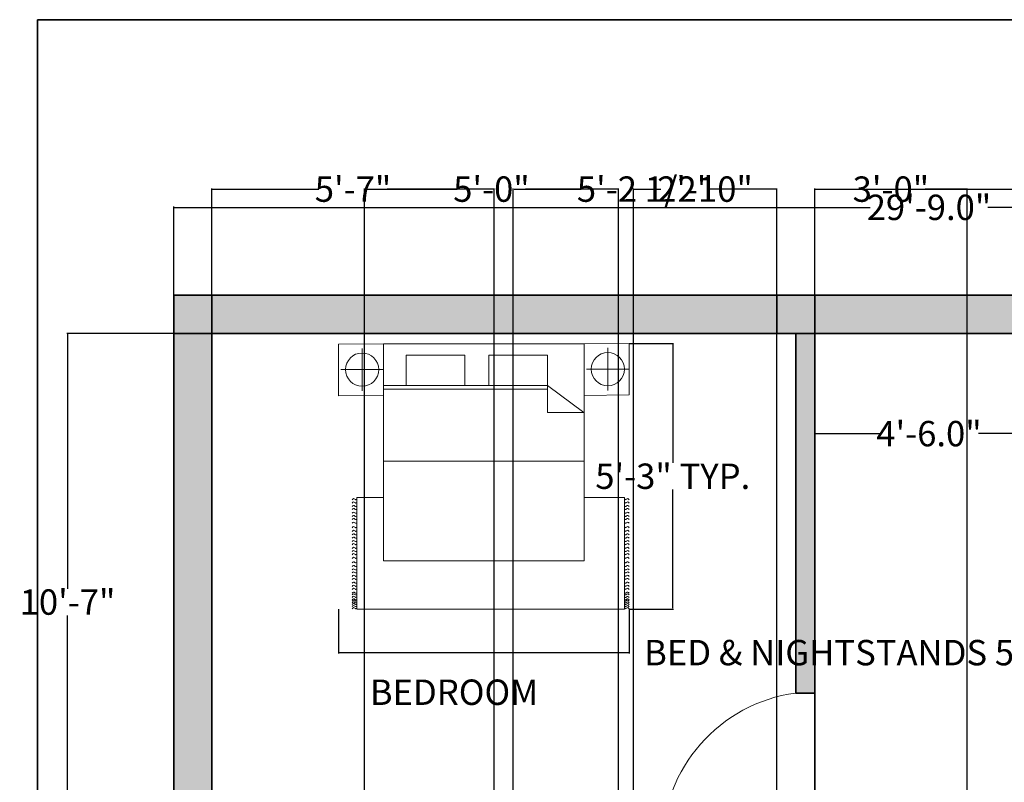
# Model space of a CAD drawing. Units: inches. Extents: x 74 to 548, y 68 to 649.
# Tile 5 of 6: x 79 to 311, y 469 to 649. Entities that reach past the tile are written whole.
import ezdxf

# ---------------------------------------------------------------- set-up
doc = ezdxf.new("R2010")
doc.units = ezdxf.units.IN
doc.header["$MEASUREMENT"] = 0
for name, color, linetype, lineweight in [('A-ANNO-DIMS', 2, 'Continuous', 18), ('A-ANNO-TTLB', 7, 'Continuous', 35), ('A-AREA-IDEN', 7, 'Continuous', 25), ('A-COLS', 7, 'Continuous', 35), ('A-DOOR', 3, 'Continuous', 18), ('A-FURN', 8, 'Continuous', 18), ('A-WALL', 7, 'Continuous', 35)]:
    doc.layers.add(name, color=color, linetype=linetype, lineweight=lineweight)
doc.layers.add('A-COLS-PATT', color=11, linetype='Continuous', lineweight=13, true_color=0xf27172)
doc.layers.add('A-WALL-PATT', color=7, linetype='Continuous', lineweight=13, true_color=0xffffff)
doc.styles.get("Standard").update_dxf_attribs({"font": 'arial.ttf'})
doc.dimstyles.get("Standard").update_dxf_attribs({"dimtxt": 6, "dimasz": 0.18, "dimexe": 0.18, "dimexo": 0.0625, "dimgap": 0.09, "dimtad": 0, "dimtih": 1, "dimtoh": 1, "dimdec": 1, "dimzin": 0, "dimdsep": 46, "dimlunit": 3, "dimtxsty": 'Standard', "dimcen": 0.09, "dimadec": 0, "dimazin": 0, "dimtfac": 1, "dimtdec": 1, "dimtofl": 0, "dimtmove": 0, "dimatfit": 3, "dimfxl": 1, "dimtolj": 1, "dimtzin": 0, "dimarcsym": 0})

# ---------------------------------------------------------------- blocks, each defined once
blk = doc.blocks.new('*D3')
at = {"layer": 'A-ANNO-DIMS', "color": 0, "lineweight": -2, "transparency": 16777216}
for p, q in [((114.96, 584.31), (114.96, 605.21)), ((471.96, 584.31), (471.96, 605.21)), ((115.14, 605.03), (279.52, 605.03)), ((471.78, 605.03), (307.4, 605.03))]:
    blk.add_line(p, q, dxfattribs=at)
at = {"layer": 'A-ANNO-DIMS', "color": 0, "transparency": 16777216}
for points in [[(115.14, 605.06), (115.14, 605), (114.96, 605.03)], [(471.78, 605.06), (471.78, 605), (471.96, 605.03)]]:
    blk.add_solid(points, dxfattribs=at)
at = {"layer": 'Defpoints', "color": 0, "transparency": 16777216}
for p in [(471.96, 605.03), (114.96, 584.24), (471.96, 584.24)]:
    blk.add_point(p, dxfattribs=at)
at = {"layer": 'A-ANNO-DIMS', "color": 0, "transparency": 16777216, "insert": (293.46, 605.03), "char_height": 6, "attachment_point": 5}
blk.add_mtext('\\A1;29\'-9.0"', dxfattribs=at)
blk = doc.blocks.new('*D5')
at = {"layer": 'A-ANNO-DIMS', "color": 0, "lineweight": -2, "transparency": 16777216}
for p, q in [((266.46, 561.7), (266.46, 551.37)), ((320.46, 559.19), (320.46, 551.37)), ((266.64, 551.55), (281.78, 551.55)), ((320.28, 551.55), (305.14, 551.55))]:
    blk.add_line(p, q, dxfattribs=at)
at = {"layer": 'A-ANNO-DIMS', "color": 0, "transparency": 16777216}
for points in [[(266.64, 551.58), (266.64, 551.52), (266.46, 551.55)], [(320.28, 551.58), (320.28, 551.52), (320.46, 551.55)]]:
    blk.add_solid(points, dxfattribs=at)
at = {"layer": 'Defpoints', "color": 0, "transparency": 16777216}
for p in [(266.46, 561.76), (320.46, 559.25), (320.46, 551.55)]:
    blk.add_point(p, dxfattribs=at)
at = {"layer": 'A-ANNO-DIMS', "color": 0, "transparency": 16777216, "insert": (293.46, 551.55), "char_height": 6, "attachment_point": 5}
blk.add_mtext('\\A1;4\'-6.0"', dxfattribs=at)
blk = doc.blocks.new('BED-DOUBLE-NIGHTSTANDS')
for p, q in [((-5.03, -1.07), (-5.03, -11.12)), ((53.03, -0.96), (53.03, -11.02)), ((0, -6.09), (-10.05, -6.09)), ((58.05, -5.99), (48, -5.99)), ((38.76, -9.86), (0, -9.86)), ((38.82, -10.68), (0, -10.68)), ((38.76, -9.86), (47.38, -16.22)), ((38.82, -9.86), (38.82, -16.22)), ((38.82, -16.22), (47.38, -16.22)), ((47.43, -27.72), (0, -27.72)), ((-6.27, -62.68), (-6.27, -36.31)), ((-6.27, -36.31), (0.03, -36.31)), ((47.43, -36.31), (56.97, -36.31)), ((56.97, -36.31), (56.97, -62.68)), ((56.97, -62.68), (-6.27, -62.68))]:
    blk.add_line(p, q)
for points in [[(-10.63, -12.29), (0, -12.19), (0, 0), (-10.63, -0.1)], [(47.43, 0), (47.43, -51.32), (0, -51.32), (0, 0)], [(47.43, -12.19), (58.05, -12.08), (58.05, 0.1), (47.43, 0)], [(19.25, -2.7), (19.25, -9.86), (5.36, -9.86), (5.36, -2.7)], [(38.82, -2.7), (38.82, -9.86), (24.92, -9.86), (24.92, -2.7)]]:
    blk.add_lwpolyline(points, close=True)
for centre in [(-5.03, -6.09), (53.03, -5.99)]:
    blk.add_circle(centre, 3.92)
for points, knots in [([(-7.4, -36.85), (-7.3, -36.72), (-7.11, -36.49), (-6.77, -36.72), (-6.49, -36.9), (-6.34, -36.79), (-6.27, -36.74)], [0, 0, 0, 0, 0.400747, 0.791423, 1.067667, 1.29709, 1.29709, 1.29709, 1.29709]), ([(58.08, -36.85), (57.99, -36.72), (57.8, -36.49), (57.45, -36.72), (57.17, -36.9), (57.02, -36.79), (56.96, -36.74)], [0, 0, 0, 0, 0.400747, 0.791423, 1.067667, 1.29709, 1.29709, 1.29709, 1.29709]), ([(-7.4, -37.62), (-7.3, -37.5), (-7.11, -37.26), (-6.77, -37.5), (-6.49, -37.68), (-6.34, -37.57), (-6.27, -37.52)], [0, 0, 0, 0, 0.400747, 0.791423, 1.067667, 1.29709, 1.29709, 1.29709, 1.29709]), ([(-7.4, -38.44), (-7.3, -38.32), (-7.11, -38.08), (-6.77, -38.32), (-6.49, -38.49), (-6.34, -38.39), (-6.27, -38.34)], [0, 0, 0, 0, 0.400747, 0.791423, 1.067667, 1.29709, 1.29709, 1.29709, 1.29709]), ([(-7.4, -39.17), (-7.3, -39.05), (-7.11, -38.81), (-6.77, -39.05), (-6.49, -39.22), (-6.34, -39.11), (-6.27, -39.07)], [0, 0, 0, 0, 0.400747, 0.791423, 1.067667, 1.29709, 1.29709, 1.29709, 1.29709]), ([(58.08, -37.62), (57.99, -37.5), (57.8, -37.26), (57.45, -37.5), (57.17, -37.68), (57.02, -37.57), (56.96, -37.52)], [0, 0, 0, 0, 0.400747, 0.791423, 1.067667, 1.29709, 1.29709, 1.29709, 1.29709]), ([(58.08, -38.44), (57.99, -38.32), (57.8, -38.08), (57.45, -38.32), (57.17, -38.49), (57.02, -38.39), (56.96, -38.34)], [0, 0, 0, 0, 0.400747, 0.791423, 1.067667, 1.29709, 1.29709, 1.29709, 1.29709]), ([(58.08, -39.17), (57.99, -39.05), (57.8, -38.81), (57.45, -39.05), (57.17, -39.22), (57.02, -39.11), (56.96, -39.07)], [0, 0, 0, 0, 0.400747, 0.791423, 1.067667, 1.29709, 1.29709, 1.29709, 1.29709]), ([(-7.4, -40.05), (-7.3, -39.93), (-7.11, -39.69), (-6.77, -39.93), (-6.49, -40.1), (-6.34, -40), (-6.27, -39.95)], [0, 0, 0, 0, 0.400747, 0.791423, 1.067667, 1.29709, 1.29709, 1.29709, 1.29709]), ([(-7.4, -40.8), (-7.3, -40.68), (-7.11, -40.44), (-6.77, -40.68), (-6.49, -40.85), (-6.34, -40.75), (-6.27, -40.7)], [0, 0, 0, 0, 0.400747, 0.791423, 1.067667, 1.29709, 1.29709, 1.29709, 1.29709]), ([(-7.4, -41.53), (-7.3, -41.41), (-7.11, -41.17), (-6.77, -41.41), (-6.49, -41.58), (-6.34, -41.48), (-6.27, -41.43)], [0, 0, 0, 0, 0.400747, 0.791423, 1.067667, 1.29709, 1.29709, 1.29709, 1.29709]), ([(58.08, -40.05), (57.99, -39.93), (57.8, -39.69), (57.45, -39.93), (57.17, -40.1), (57.02, -40), (56.96, -39.95)], [0, 0, 0, 0, 0.400747, 0.791423, 1.067667, 1.29709, 1.29709, 1.29709, 1.29709]), ([(58.08, -40.8), (57.99, -40.68), (57.8, -40.44), (57.45, -40.68), (57.17, -40.85), (57.02, -40.75), (56.96, -40.7)], [0, 0, 0, 0, 0.400747, 0.791423, 1.067667, 1.29709, 1.29709, 1.29709, 1.29709]), ([(58.08, -41.53), (57.99, -41.41), (57.8, -41.17), (57.45, -41.41), (57.17, -41.58), (57.02, -41.48), (56.96, -41.43)], [0, 0, 0, 0, 0.400747, 0.791423, 1.067667, 1.29709, 1.29709, 1.29709, 1.29709]), ([(-7.4, -42.41), (-7.3, -42.29), (-7.11, -42.05), (-6.77, -42.29), (-6.49, -42.46), (-6.34, -42.36), (-6.27, -42.31)], [0, 0, 0, 0, 0.400747, 0.791423, 1.067667, 1.29709, 1.29709, 1.29709, 1.29709]), ([(-7.4, -43.45), (-7.3, -43.33), (-7.11, -43.09), (-6.77, -43.33), (-6.49, -43.5), (-6.34, -43.39), (-6.27, -43.35)], [0, 0, 0, 0, 0.400747, 0.791423, 1.067667, 1.29709, 1.29709, 1.29709, 1.29709]), ([(-7.4, -44.33), (-7.3, -44.21), (-7.11, -43.97), (-6.77, -44.21), (-6.49, -44.38), (-6.34, -44.28), (-6.27, -44.23)], [0, 0, 0, 0, 0.400747, 0.791423, 1.067667, 1.29709, 1.29709, 1.29709, 1.29709]), ([(58.08, -42.41), (57.99, -42.29), (57.8, -42.05), (57.45, -42.29), (57.17, -42.46), (57.02, -42.36), (56.96, -42.31)], [0, 0, 0, 0, 0.400747, 0.791423, 1.067667, 1.29709, 1.29709, 1.29709, 1.29709]), ([(58.08, -43.45), (57.99, -43.33), (57.8, -43.09), (57.45, -43.33), (57.17, -43.5), (57.02, -43.39), (56.96, -43.35)], [0, 0, 0, 0, 0.400747, 0.791423, 1.067667, 1.29709, 1.29709, 1.29709, 1.29709]), ([(58.08, -44.33), (57.99, -44.21), (57.8, -43.97), (57.45, -44.21), (57.17, -44.38), (57.02, -44.28), (56.96, -44.23)], [0, 0, 0, 0, 0.400747, 0.791423, 1.067667, 1.29709, 1.29709, 1.29709, 1.29709]), ([(-7.4, -45.15), (-7.3, -45.03), (-7.11, -44.79), (-6.77, -45.03), (-6.49, -45.2), (-6.34, -45.09), (-6.27, -45.05)], [0, 0, 0, 0, 0.400747, 0.791423, 1.067667, 1.29709, 1.29709, 1.29709, 1.29709]), ([(-7.4, -45.92), (-7.3, -45.8), (-7.11, -45.56), (-6.77, -45.8), (-6.49, -45.98), (-6.34, -45.87), (-6.27, -45.82)], [0, 0, 0, 0, 0.400747, 0.791423, 1.067667, 1.29709, 1.29709, 1.29709, 1.29709]), ([(-7.4, -46.74), (-7.3, -46.62), (-7.11, -46.38), (-6.77, -46.62), (-6.49, -46.79), (-6.34, -46.69), (-6.27, -46.64)], [0, 0, 0, 0, 0.400747, 0.791423, 1.067667, 1.29709, 1.29709, 1.29709, 1.29709]), ([(58.08, -45.15), (57.99, -45.03), (57.8, -44.79), (57.45, -45.03), (57.17, -45.2), (57.02, -45.09), (56.96, -45.05)], [0, 0, 0, 0, 0.400747, 0.791423, 1.067667, 1.29709, 1.29709, 1.29709, 1.29709]), ([(58.08, -45.92), (57.99, -45.8), (57.8, -45.56), (57.45, -45.8), (57.17, -45.98), (57.02, -45.87), (56.96, -45.82)], [0, 0, 0, 0, 0.400747, 0.791423, 1.067667, 1.29709, 1.29709, 1.29709, 1.29709]), ([(58.08, -46.74), (57.99, -46.62), (57.8, -46.38), (57.45, -46.62), (57.17, -46.79), (57.02, -46.69), (56.96, -46.64)], [0, 0, 0, 0, 0.400747, 0.791423, 1.067667, 1.29709, 1.29709, 1.29709, 1.29709]), ([(-7.4, -47.47), (-7.3, -47.35), (-7.11, -47.11), (-6.77, -47.35), (-6.49, -47.52), (-6.34, -47.41), (-6.27, -47.37)], [0, 0, 0, 0, 0.400747, 0.791423, 1.067667, 1.29709, 1.29709, 1.29709, 1.29709]), ([(-7.4, -48.35), (-7.3, -48.23), (-7.11, -47.99), (-6.77, -48.23), (-6.49, -48.4), (-6.34, -48.3), (-6.27, -48.25)], [0, 0, 0, 0, 0.400747, 0.791423, 1.067667, 1.29709, 1.29709, 1.29709, 1.29709]), ([(-7.4, -49.1), (-7.3, -48.98), (-7.11, -48.74), (-6.77, -48.98), (-6.49, -49.15), (-6.34, -49.05), (-6.27, -49)], [0, 0, 0, 0, 0.400747, 0.791423, 1.067667, 1.29709, 1.29709, 1.29709, 1.29709]), ([(58.08, -47.47), (57.99, -47.35), (57.8, -47.11), (57.45, -47.35), (57.17, -47.52), (57.02, -47.41), (56.96, -47.37)], [0, 0, 0, 0, 0.400747, 0.791423, 1.067667, 1.29709, 1.29709, 1.29709, 1.29709]), ([(58.08, -48.35), (57.99, -48.23), (57.8, -47.99), (57.45, -48.23), (57.17, -48.4), (57.02, -48.3), (56.96, -48.25)], [0, 0, 0, 0, 0.400747, 0.791423, 1.067667, 1.29709, 1.29709, 1.29709, 1.29709]), ([(58.08, -49.1), (57.99, -48.98), (57.8, -48.74), (57.45, -48.98), (57.17, -49.15), (57.02, -49.05), (56.96, -49)], [0, 0, 0, 0, 0.400747, 0.791423, 1.067667, 1.29709, 1.29709, 1.29709, 1.29709]), ([(-7.4, -49.83), (-7.3, -49.71), (-7.11, -49.47), (-6.77, -49.71), (-6.49, -49.88), (-6.34, -49.78), (-6.27, -49.73)], [0, 0, 0, 0, 0.400747, 0.791423, 1.067667, 1.29709, 1.29709, 1.29709, 1.29709]), ([(-7.4, -50.71), (-7.3, -50.59), (-7.11, -50.35), (-6.77, -50.59), (-6.49, -50.77), (-6.34, -50.66), (-6.27, -50.61)], [0, 0, 0, 0, 0.400747, 0.791423, 1.067667, 1.29709, 1.29709, 1.29709, 1.29709]), ([(58.08, -49.83), (57.99, -49.71), (57.8, -49.47), (57.45, -49.71), (57.17, -49.88), (57.02, -49.78), (56.96, -49.73)], [0, 0, 0, 0, 0.400747, 0.791423, 1.067667, 1.29709, 1.29709, 1.29709, 1.29709]), ([(58.08, -50.71), (57.99, -50.59), (57.8, -50.35), (57.45, -50.59), (57.17, -50.77), (57.02, -50.66), (56.96, -50.61)], [0, 0, 0, 0, 0.400747, 0.791423, 1.067667, 1.29709, 1.29709, 1.29709, 1.29709]), ([(-7.4, -51.75), (-7.3, -51.63), (-7.11, -51.39), (-6.77, -51.63), (-6.49, -51.8), (-6.34, -51.7), (-6.27, -51.65)], [0, 0, 0, 0, 0.400747, 0.791423, 1.067667, 1.29709, 1.29709, 1.29709, 1.29709]), ([(-7.4, -52.63), (-7.3, -52.51), (-7.11, -52.27), (-6.77, -52.51), (-6.49, -52.68), (-6.34, -52.58), (-6.27, -52.53)], [0, 0, 0, 0, 0.400747, 0.791423, 1.067667, 1.29709, 1.29709, 1.29709, 1.29709]), ([(-7.4, -53.45), (-7.3, -53.33), (-7.11, -53.09), (-6.77, -53.33), (-6.49, -53.5), (-6.34, -53.39), (-6.27, -53.35)], [0, 0, 0, 0, 0.400747, 0.791423, 1.067667, 1.29709, 1.29709, 1.29709, 1.29709]), ([(58.08, -51.75), (57.99, -51.63), (57.8, -51.39), (57.45, -51.63), (57.17, -51.8), (57.02, -51.7), (56.96, -51.65)], [0, 0, 0, 0, 0.400747, 0.791423, 1.067667, 1.29709, 1.29709, 1.29709, 1.29709]), ([(58.08, -52.63), (57.99, -52.51), (57.8, -52.27), (57.45, -52.51), (57.17, -52.68), (57.02, -52.58), (56.96, -52.53)], [0, 0, 0, 0, 0.400747, 0.791423, 1.067667, 1.29709, 1.29709, 1.29709, 1.29709]), ([(58.08, -53.45), (57.99, -53.33), (57.8, -53.09), (57.45, -53.33), (57.17, -53.5), (57.02, -53.39), (56.96, -53.35)], [0, 0, 0, 0, 0.400747, 0.791423, 1.067667, 1.29709, 1.29709, 1.29709, 1.29709]), ([(-7.4, -54.14), (-7.3, -54.02), (-7.11, -53.78), (-6.77, -54.02), (-6.49, -54.19), (-6.34, -54.08), (-6.27, -54.04)], [0, 0, 0, 0, 0.400747, 0.791423, 1.067667, 1.29709, 1.29709, 1.29709, 1.29709]), ([(-7.4, -54.95), (-7.3, -54.83), (-7.11, -54.59), (-6.77, -54.83), (-6.49, -55.01), (-6.34, -54.9), (-6.27, -54.85)], [0, 0, 0, 0, 0.400747, 0.791423, 1.067667, 1.29709, 1.29709, 1.29709, 1.29709]), ([(-7.4, -55.68), (-7.3, -55.56), (-7.11, -55.32), (-6.77, -55.56), (-6.49, -55.73), (-6.34, -55.63), (-6.27, -55.58)], [0, 0, 0, 0, 0.400747, 0.791423, 1.067667, 1.29709, 1.29709, 1.29709, 1.29709]), ([(58.08, -54.14), (57.99, -54.02), (57.8, -53.78), (57.45, -54.02), (57.17, -54.19), (57.02, -54.08), (56.96, -54.04)], [0, 0, 0, 0, 0.400747, 0.791423, 1.067667, 1.29709, 1.29709, 1.29709, 1.29709]), ([(58.08, -54.95), (57.99, -54.83), (57.8, -54.59), (57.45, -54.83), (57.17, -55.01), (57.02, -54.9), (56.96, -54.85)], [0, 0, 0, 0, 0.400747, 0.791423, 1.067667, 1.29709, 1.29709, 1.29709, 1.29709]), ([(58.08, -55.68), (57.99, -55.56), (57.8, -55.32), (57.45, -55.56), (57.17, -55.73), (57.02, -55.63), (56.96, -55.58)], [0, 0, 0, 0, 0.400747, 0.791423, 1.067667, 1.29709, 1.29709, 1.29709, 1.29709]), ([(-7.4, -56.56), (-7.3, -56.44), (-7.11, -56.2), (-6.77, -56.44), (-6.49, -56.62), (-6.34, -56.51), (-6.27, -56.46)], [0, 0, 0, 0, 0.400747, 0.791423, 1.067667, 1.29709, 1.29709, 1.29709, 1.29709]), ([(-7.4, -57.32), (-7.3, -57.2), (-7.11, -56.96), (-6.77, -57.2), (-6.49, -57.37), (-6.34, -57.26), (-6.27, -57.21)], [0, 0, 0, 0, 0.400747, 0.791423, 1.067667, 1.29709, 1.29709, 1.29709, 1.29709]), ([(-7.4, -58.04), (-7.3, -57.92), (-7.11, -57.68), (-6.77, -57.92), (-6.49, -58.1), (-6.34, -57.99), (-6.27, -57.94)], [0, 0, 0, 0, 0.400747, 0.791423, 1.067667, 1.29709, 1.29709, 1.29709, 1.29709]), ([(58.08, -56.56), (57.99, -56.44), (57.8, -56.2), (57.45, -56.44), (57.17, -56.62), (57.02, -56.51), (56.96, -56.46)], [0, 0, 0, 0, 0.400747, 0.791423, 1.067667, 1.29709, 1.29709, 1.29709, 1.29709]), ([(58.08, -57.32), (57.99, -57.2), (57.8, -56.96), (57.45, -57.2), (57.17, -57.37), (57.02, -57.26), (56.96, -57.21)], [0, 0, 0, 0, 0.400747, 0.791423, 1.067667, 1.29709, 1.29709, 1.29709, 1.29709]), ([(58.08, -58.04), (57.99, -57.92), (57.8, -57.68), (57.45, -57.92), (57.18, -58.09), (57.03, -57.99), (56.97, -57.95)], [0, 0, 0, 0, 0.400747, 0.791423, 1.067667, 1.283686, 1.283686, 1.283686, 1.283686]), ([(-7.4, -58.93), (-7.3, -58.81), (-7.11, -58.57), (-6.77, -58.81), (-6.49, -58.98), (-6.34, -58.87), (-6.27, -58.82)], [0, 0, 0, 0, 0.400747, 0.791423, 1.067667, 1.29709, 1.29709, 1.29709, 1.29709]), ([(-7.4, -59.36), (-7.3, -59.23), (-7.11, -58.98), (-6.77, -59.24), (-6.49, -59.41), (-6.34, -59.3), (-6.27, -59.25)], [0, 0, 0, 0, 0.407265, 0.802015, 1.07826, 1.307683, 1.307683, 1.307683, 1.307683]), ([(-7.4, -59.92), (-7.3, -59.8), (-7.11, -59.56), (-6.77, -59.8), (-6.49, -59.97), (-6.34, -59.87), (-6.27, -59.82)], [0, 0, 0, 0, 0.400747, 0.791423, 1.067667, 1.29709, 1.29709, 1.29709, 1.29709]), ([(-7.4, -60.5), (-7.3, -60.38), (-7.11, -60.14), (-6.77, -60.38), (-6.49, -60.55), (-6.34, -60.44), (-6.27, -60.39)], [0, 0, 0, 0, 0.400747, 0.791423, 1.067667, 1.29709, 1.29709, 1.29709, 1.29709]), ([(58.08, -58.93), (57.99, -58.81), (57.8, -58.57), (57.45, -58.81), (57.18, -58.98), (57.03, -58.88), (56.97, -58.83)], [0, 0, 0, 0, 0.400747, 0.791423, 1.067667, 1.283686, 1.283686, 1.283686, 1.283686]), ([(58.08, -59.36), (57.99, -59.23), (57.8, -58.99), (57.45, -59.24), (57.18, -59.41), (57.03, -59.31), (56.97, -59.26)], [0, 0, 0, 0, 0.402903, 0.794912, 1.071156, 1.287177, 1.287177, 1.287177, 1.287177]), ([(58.08, -59.95), (57.99, -59.83), (57.8, -59.59), (57.45, -59.83), (57.18, -60), (57.03, -59.9), (56.97, -59.86)], [0, 0, 0, 0, 0.400747, 0.791423, 1.067667, 1.283686, 1.283686, 1.283686, 1.283686]), ([(58.08, -60.52), (57.99, -60.4), (57.8, -60.16), (57.45, -60.4), (57.18, -60.57), (57.03, -60.47), (56.97, -60.43)], [0, 0, 0, 0, 0.400747, 0.791423, 1.067667, 1.283686, 1.283686, 1.283686, 1.283686]), ([(-7.4, -60.81), (-7.3, -60.68), (-7.11, -60.44), (-6.77, -60.68), (-6.49, -60.86), (-6.34, -60.75), (-6.27, -60.7)], [0, 0, 0, 0, 0.400747, 0.791423, 1.067667, 1.29709, 1.29709, 1.29709, 1.29709]), ([(-7.4, -61.22), (-7.3, -61.1), (-7.11, -60.86), (-6.77, -61.1), (-6.49, -61.28), (-6.34, -61.17), (-6.27, -61.12)], [0, 0, 0, 0, 0.400747, 0.791423, 1.067667, 1.29709, 1.29709, 1.29709, 1.29709]), ([(-7.4, -61.62), (-7.3, -61.5), (-7.11, -61.26), (-6.77, -61.5), (-6.49, -61.67), (-6.34, -61.57), (-6.27, -61.52)], [0, 0, 0, 0, 0.400747, 0.791423, 1.067667, 1.29709, 1.29709, 1.29709, 1.29709]), ([(-7.4, -62.11), (-7.3, -61.99), (-7.11, -61.75), (-6.77, -61.99), (-6.49, -62.16), (-6.34, -62.05), (-6.27, -62)], [0, 0, 0, 0, 0.400747, 0.791423, 1.067667, 1.29709, 1.29709, 1.29709, 1.29709]), ([(-7.4, -62.61), (-7.3, -62.49), (-7.11, -62.25), (-6.77, -62.49), (-6.49, -62.66), (-6.34, -62.55), (-6.27, -62.51)], [0, 0, 0, 0, 0.400747, 0.791423, 1.067667, 1.29709, 1.29709, 1.29709, 1.29709]), ([(58.08, -61.25), (57.99, -61.13), (57.8, -60.89), (57.45, -61.13), (57.17, -61.3), (57.02, -61.2), (56.96, -61.15)], [0, 0, 0, 0, 0.400747, 0.791423, 1.067667, 1.29709, 1.29709, 1.29709, 1.29709]), ([(58.08, -61.65), (57.99, -61.53), (57.8, -61.29), (57.45, -61.53), (57.17, -61.7), (57.02, -61.6), (56.96, -61.55)], [0, 0, 0, 0, 0.400747, 0.791423, 1.067667, 1.29709, 1.29709, 1.29709, 1.29709]), ([(58.08, -62.13), (57.99, -62.01), (57.8, -61.77), (57.45, -62.01), (57.17, -62.19), (57.02, -62.08), (56.96, -62.03)], [0, 0, 0, 0, 0.400747, 0.791423, 1.067667, 1.29709, 1.29709, 1.29709, 1.29709]), ([(58.08, -62.61), (57.99, -62.49), (57.8, -62.25), (57.45, -62.49), (57.17, -62.66), (57.02, -62.55), (56.96, -62.51)], [0, 0, 0, 0, 0.400747, 0.791423, 1.067667, 1.29709, 1.29709, 1.29709, 1.29709]), ([(58.08, -60.83), (57.99, -60.71), (57.8, -60.47), (57.45, -60.71), (57.18, -60.88), (57.03, -60.78), (56.97, -60.74)], [0, 0, 0, 0, 0.400747, 0.791423, 1.067667, 1.283686, 1.283686, 1.283686, 1.283686])]:
    blk.add_open_spline(points, degree=3, knots=knots)
blk = doc.blocks.new('DOOR-SWING-36IN')
for p, q in [((0, 0), (0, 36)), ((-36, 1), (0, 1)), ((0, 0), (-36, 0))]:
    blk.add_line(p, q)
blk.add_arc((0.32, 0), 36.32, 97.6281, 180)
blk = doc.blocks.new('*D12')
at = {"layer": 'A-ANNO-DIMS', "color": 0, "lineweight": -2, "transparency": 16777216}
for p, q in [((153.88, 510.03), (153.88, 499.61)), ((222.59, 510.03), (222.59, 499.61)), ((154.06, 499.79), (222.41, 499.79)), ((222.59, 499.79), (222.77, 499.79))]:
    blk.add_line(p, q, dxfattribs=at)
at = {"layer": 'A-ANNO-DIMS', "color": 0, "transparency": 16777216}
for points in [[(154.06, 499.82), (154.06, 499.76), (153.88, 499.79)], [(222.41, 499.82), (222.41, 499.76), (222.59, 499.79)]]:
    blk.add_solid(points, dxfattribs=at)
at = {"layer": 'Defpoints', "color": 0, "transparency": 16777216}
for p in [(153.88, 510.09), (222.59, 510.09), (222.59, 499.79)]:
    blk.add_point(p, dxfattribs=at)
at = {"layer": 'A-ANNO-DIMS', "color": 0, "transparency": 16777216, "insert": (292.95, 499.79), "char_height": 6, "attachment_point": 5}
blk.add_mtext('\\A1;BED & NIGHTSTANDS 5\'-8 1/2" TYP.', dxfattribs=at)
blk = doc.blocks.new('*D13')
at = {"layer": 'A-ANNO-DIMS', "color": 0, "lineweight": -2, "transparency": 16777216}
for p, q in [((222.65, 572.88), (233.08, 572.88)), ((232.9, 572.7), (232.9, 544.64)), ((232.9, 510.27), (232.9, 538.33)), ((222.65, 510.09), (233.08, 510.09))]:
    blk.add_line(p, q, dxfattribs=at)
at = {"layer": 'A-ANNO-DIMS', "color": 0, "transparency": 16777216}
for points in [[(232.87, 572.7), (232.93, 572.7), (232.9, 572.88)], [(232.87, 510.27), (232.93, 510.27), (232.9, 510.09)]]:
    blk.add_solid(points, dxfattribs=at)
at = {"layer": 'Defpoints', "color": 0, "transparency": 16777216}
for p in [(222.59, 572.88), (232.9, 572.88), (222.59, 510.09)]:
    blk.add_point(p, dxfattribs=at)
at = {"layer": 'A-ANNO-DIMS', "color": 0, "transparency": 16777216, "insert": (232.9, 541.48), "char_height": 6, "attachment_point": 5}
blk.add_mtext('\\A1;5\'-3" TYP.', dxfattribs=at)
blk = doc.blocks.new('*D18')
at = {"layer": 'A-ANNO-DIMS', "color": 0, "lineweight": -2, "transparency": 16777216}
for p, q in [((114.9, 575.24), (89.68, 575.24)), ((89.86, 575.06), (89.86, 514.9)), ((89.86, 448.42), (89.86, 508.59)), ((123.9, 448.24), (89.68, 448.24))]:
    blk.add_line(p, q, dxfattribs=at)
at = {"layer": 'A-ANNO-DIMS', "color": 0, "transparency": 16777216}
for points in [[(89.83, 575.06), (89.89, 575.06), (89.86, 575.24)], [(89.83, 448.42), (89.89, 448.42), (89.86, 448.24)]]:
    blk.add_solid(points, dxfattribs=at)
at = {"layer": 'Defpoints', "color": 0, "transparency": 16777216}
for p in [(89.86, 575.24), (114.96, 575.24), (123.96, 448.24)]:
    blk.add_point(p, dxfattribs=at)
at = {"layer": 'A-ANNO-DIMS', "color": 0, "transparency": 16777216, "insert": (89.86, 511.74), "char_height": 6, "attachment_point": 5}
blk.add_mtext('\\A1;10\'-7"', dxfattribs=at)
blk = doc.blocks.new('*D19')
at = {"layer": 'A-ANNO-DIMS', "color": 0, "lineweight": -2, "transparency": 16777216}
for p, q in [((123.96, 361.31), (123.96, 609.52)), ((124.14, 609.34), (149.27, 609.34)), ((190.53, 609.34), (165.4, 609.34)), ((190.71, 365.81), (190.71, 609.52))]:
    blk.add_line(p, q, dxfattribs=at)
at = {"layer": 'A-ANNO-DIMS', "color": 0, "transparency": 16777216}
for points in [[(124.14, 609.37), (124.14, 609.31), (123.96, 609.34)], [(190.53, 609.37), (190.53, 609.31), (190.71, 609.34)]]:
    blk.add_solid(points, dxfattribs=at)
at = {"layer": 'Defpoints', "color": 0, "transparency": 16777216}
for p in [(190.71, 609.34), (190.71, 365.74), (123.96, 361.24)]:
    blk.add_point(p, dxfattribs=at)
at = {"layer": 'A-ANNO-DIMS', "color": 0, "transparency": 16777216, "insert": (157.34, 609.34), "char_height": 6, "attachment_point": 5}
blk.add_mtext('\\A1;5\'-7"', dxfattribs=at)
blk = doc.blocks.new('*D20')
at = {"layer": 'A-ANNO-DIMS', "color": 0, "lineweight": -2, "transparency": 16777216}
for p, q in [((195.21, 365.81), (195.21, 609.52)), ((195.39, 609.34), (211.28, 609.34)), ((257.28, 609.34), (241.39, 609.34)), ((257.46, 365.81), (257.46, 609.52))]:
    blk.add_line(p, q, dxfattribs=at)
at = {"layer": 'A-ANNO-DIMS', "color": 0, "transparency": 16777216}
for points in [[(195.39, 609.37), (195.39, 609.31), (195.21, 609.34)], [(257.28, 609.37), (257.28, 609.31), (257.46, 609.34)]]:
    blk.add_solid(points, dxfattribs=at)
at = {"layer": 'Defpoints', "color": 0, "transparency": 16777216}
for p in [(257.46, 609.34), (195.21, 365.74), (257.46, 365.74)]:
    blk.add_point(p, dxfattribs=at)
at = {"layer": 'A-ANNO-DIMS', "color": 0, "transparency": 16777216, "insert": (226.34, 609.34), "char_height": 6, "attachment_point": 5}
blk.add_mtext('\\A1;5\'-2 1/2"', dxfattribs=at)
blk = doc.blocks.new('*D30')
at = {"layer": 'A-ANNO-DIMS', "color": 0, "lineweight": -2, "transparency": 16777216}
for p, q in [((160.05, 220.81), (160.05, 609.52)), ((160.23, 609.34), (181.98, 609.34)), ((219.87, 609.34), (198.11, 609.34)), ((220.05, 220.81), (220.05, 609.52))]:
    blk.add_line(p, q, dxfattribs=at)
at = {"layer": 'A-ANNO-DIMS', "color": 0, "transparency": 16777216}
for points in [[(160.23, 609.37), (160.23, 609.31), (160.05, 609.34)], [(219.87, 609.37), (219.87, 609.31), (220.05, 609.34)]]:
    blk.add_solid(points, dxfattribs=at)
at = {"layer": 'Defpoints', "color": 0, "transparency": 16777216}
for p in [(220.05, 609.34), (160.05, 220.74), (220.05, 220.74)]:
    blk.add_point(p, dxfattribs=at)
at = {"layer": 'A-ANNO-DIMS', "color": 0, "transparency": 16777216, "insert": (190.05, 609.34), "char_height": 6, "attachment_point": 5}
blk.add_mtext('\\A1;5\'-0"', dxfattribs=at)
blk = doc.blocks.new('*D36')
at = {"layer": 'A-ANNO-DIMS', "color": 0, "lineweight": -2, "transparency": 16777216}
for p, q in [((266.46, 223.31), (266.46, 609.52)), ((266.64, 609.34), (276.4, 609.34)), ((302.28, 609.34), (292.52, 609.34)), ((302.46, 223.31), (302.46, 609.52))]:
    blk.add_line(p, q, dxfattribs=at)
at = {"layer": 'A-ANNO-DIMS', "color": 0, "transparency": 16777216}
for points in [[(266.64, 609.37), (266.64, 609.31), (266.46, 609.34)], [(302.28, 609.37), (302.28, 609.31), (302.46, 609.34)]]:
    blk.add_solid(points, dxfattribs=at)
at = {"layer": 'Defpoints', "color": 0, "transparency": 16777216}
for p in [(302.46, 609.34), (266.46, 223.24), (302.46, 223.24)]:
    blk.add_point(p, dxfattribs=at)
at = {"layer": 'A-ANNO-DIMS', "color": 0, "transparency": 16777216, "insert": (284.46, 609.34), "char_height": 6, "attachment_point": 5}
blk.add_mtext('\\A1;3\'-0"', dxfattribs=at)
blk = doc.blocks.new('*D37')
at = {"layer": 'A-ANNO-DIMS', "color": 0, "lineweight": -2, "transparency": 16777216}
for p, q in [((266.46, 297.87), (266.46, 609.52)), ((266.64, 609.34), (322.83, 609.34)), ((399.25, 609.34), (343.06, 609.34)), ((399.43, 299.06), (399.43, 609.52))]:
    blk.add_line(p, q, dxfattribs=at)
at = {"layer": 'A-ANNO-DIMS', "color": 0, "transparency": 16777216}
for points in [[(266.64, 609.37), (266.64, 609.31), (266.46, 609.34)], [(399.25, 609.37), (399.25, 609.31), (399.43, 609.34)]]:
    blk.add_solid(points, dxfattribs=at)
at = {"layer": 'Defpoints', "color": 0, "transparency": 16777216}
for p in [(399.43, 609.34), (399.43, 298.99), (266.46, 297.81)]:
    blk.add_point(p, dxfattribs=at)
at = {"layer": 'A-ANNO-DIMS', "color": 0, "transparency": 16777216, "insert": (332.94, 609.34), "char_height": 6, "attachment_point": 5}
blk.add_mtext('\\A1;11\'-1"', dxfattribs=at)
blk = doc.blocks.new('*D42')
at = {"layer": 'A-ANNO-DIMS', "color": 0, "lineweight": -2, "transparency": 16777216}
for p, q in [((223.59, 223.31), (223.59, 609.52)), ((223.77, 609.34), (230.08, 609.34)), ((257.28, 609.34), (250.97, 609.34)), ((257.46, 223.31), (257.46, 609.52))]:
    blk.add_line(p, q, dxfattribs=at)
at = {"layer": 'A-ANNO-DIMS', "color": 0, "transparency": 16777216}
for points in [[(223.77, 609.37), (223.77, 609.31), (223.59, 609.34)], [(257.28, 609.37), (257.28, 609.31), (257.46, 609.34)]]:
    blk.add_solid(points, dxfattribs=at)
at = {"layer": 'Defpoints', "color": 0, "transparency": 16777216}
for p in [(257.46, 609.34), (223.59, 223.24), (257.46, 223.24)]:
    blk.add_point(p, dxfattribs=at)
at = {"layer": 'A-ANNO-DIMS', "color": 0, "transparency": 16777216, "insert": (240.52, 609.34), "char_height": 6, "attachment_point": 5}
blk.add_mtext('\\A1;2\'-10"', dxfattribs=at)

msp = doc.modelspace()

# ---------------------------------------------------------------- hatches: boundary and pattern name
at = {"layer": 'A-COLS-PATT'}
h = msp.add_hatch(color=256, dxfattribs=at)
h.dxf.hatch_style = 1
h.paths.add_polyline_path([(123.96, 584.24), (114.96, 584.24), (114.96, 575.24), (123.96, 575.24)])
h.paths.add_polyline_path([(266.46, 584.24), (257.46, 584.24), (257.46, 575.24), (266.46, 575.24)])
h.paths.add_polyline_path([(329.46, 584.24), (320.46, 584.24), (320.46, 575.24), (329.46, 575.24)])
h.paths.add_polyline_path([(471.96, 584.24), (462.96, 584.24), (462.96, 575.24), (471.96, 575.24)])
h.paths.add_polyline_path([(123.96, 448.24), (114.96, 448.24), (114.96, 439.24), (123.96, 439.24)])
h.paths.add_polyline_path([(266.46, 448.24), (261.96, 448.24), (257.46, 448.24), (257.46, 439.24), (266.46, 439.24)])
h.paths.add_polyline_path([(329.46, 448.24), (320.46, 448.24), (320.46, 439.24), (329.46, 439.24)])
h.paths.add_polyline_path([(471.96, 448.24), (462.96, 448.24), (462.96, 439.24), (471.96, 439.24)])
h.paths.add_polyline_path([(123.96, 365.74), (114.96, 365.74), (114.96, 356.74), (123.96, 356.74)])
h.paths.add_polyline_path([(266.46, 365.74), (257.46, 365.74), (257.46, 356.74), (266.46, 356.74)])
h.paths.add_polyline_path([(123.96, 223.24), (114.96, 223.24), (114.96, 214.24), (123.96, 214.24)])
h.paths.add_polyline_path([(266.46, 223.24), (257.46, 223.24), (257.46, 214.24), (266.46, 214.24)])
h.paths.add_polyline_path([(123.96, 142.24), (114.96, 142.24), (114.96, 133.24), (123.96, 133.24)])
h.paths.add_polyline_path([(263.89, 142.24), (254.89, 142.24), (254.89, 133.24), (263.89, 133.24)])
h.paths.add_polyline_path([(471.96, 142.24), (462.96, 142.24), (462.96, 133.24), (471.96, 133.24)])
h.paths.add_polyline_path([(377.46, 142.24), (368.46, 142.24), (368.46, 133.24), (377.46, 133.24)])
h.paths.add_polyline_path([(377.46, 223.24), (368.46, 223.24), (368.46, 214.24), (377.46, 214.24)])
h.paths.add_polyline_path([(471.96, 223.24), (462.96, 223.24), (462.96, 214.24), (471.96, 214.24)])
h.paths.add_polyline_path([(471.96, 298.99), (462.96, 298.99), (462.96, 289.99), (471.96, 289.99)])
h.paths.add_polyline_path([(471.96, 365.74), (462.96, 365.74), (462.96, 356.74), (471.96, 356.74)])
at = {"layer": 'A-WALL-PATT'}
h = msp.add_hatch(color=256, dxfattribs=at)
h.dxf.hatch_style = 1
h.paths.add_polyline_path([(123.96, 356.74), (114.96, 356.74), (114.96, 223.24), (123.96, 223.24)])
h.paths.add_polyline_path([(123.96, 439.24), (114.96, 439.24), (114.96, 365.74), (123.96, 365.74)])
h.paths.add_polyline_path([(123.96, 575.24), (114.96, 575.24), (114.96, 448.24), (123.96, 448.24)])
h.paths.add_polyline_path([(257.46, 584.24), (123.96, 584.24), (123.96, 575.24), (257.46, 575.24)])
h.paths.add_polyline_path([(266.46, 575.24), (261.96, 575.24), (261.96, 490.24), (266.46, 490.24)])
h.paths.add_polyline_path([(266.46, 454.24), (261.96, 454.24), (261.96, 448.24), (266.46, 448.24)])
h.paths.add_polyline_path([(257.46, 448.24), (187.71, 448.24), (187.71, 443.74), (190.71, 443.74), (190.71, 365.74), (123.96, 365.74), (123.96, 361.24), (257.46, 361.24), (257.46, 365.74), (195.21, 365.74), (195.21, 443.74), (257.46, 443.74)])
h.paths.add_polyline_path([(163.71, 448.24), (123.96, 448.24), (123.96, 443.74), (163.71, 443.74)], flags=17)
h.paths.add_polyline_path([(223.59, 223.24), (220.05, 223.24), (220.05, 216.24), (160.05, 216.24), (160.05, 223.24), (123.96, 223.24), (123.96, 214.24), (159.96, 214.24), (223.59, 214.24)])
h.paths.add_polyline_path([(123.96, 214.24), (114.96, 214.24), (114.96, 142.24), (123.96, 142.24)])
h.paths.add_polyline_path([(254.89, 142.24), (123.96, 142.24), (123.96, 133.24), (254.89, 133.24)])
h.paths.add_polyline_path([(462.96, 142.24), (377.46, 142.24), (377.46, 133.24), (462.96, 133.24)])
h.paths.add_polyline_path([(372.96, 189.24), (368.46, 189.24), (368.46, 142.24), (372.96, 142.24)])
h.paths.add_polyline_path([(471.96, 214.24), (462.96, 214.24), (462.96, 142.24), (471.96, 142.24)])
h.paths.add_polyline_path([(462.96, 223.24), (403.93, 223.24), (403.93, 294.49), (409.93, 294.49), (409.93, 298.99), (403.93, 298.99), (399.43, 298.99), (399.43, 223.24), (377.46, 223.24), (377.46, 214.24), (462.96, 214.24)])
h.paths.add_polyline_path([(368.46, 223.24), (353.46, 223.24), (353.46, 216.24), (305.46, 216.24), (305.46, 223.24), (302.46, 223.24), (302.46, 214.24), (368.46, 214.24)])
h.paths.add_polyline_path([(471.96, 289.99), (462.96, 289.99), (462.96, 223.24), (471.96, 223.24)])
h.paths.add_polyline_path([(462.96, 298.99), (433.93, 298.99), (433.93, 294.49), (462.96, 294.49)], flags=0)
h.paths.add_polyline_path([(471.96, 356.74), (462.96, 356.74), (462.96, 298.99), (471.96, 298.99)])
h.paths.add_polyline_path([(462.96, 365.74), (403.93, 365.74), (403.93, 361.24), (462.96, 361.24)], flags=17)
h.paths.add_polyline_path([(471.96, 439.24), (462.96, 439.24), (462.96, 365.74), (471.96, 365.74)])
h.paths.add_polyline_path([(462.96, 448.24), (329.46, 448.24), (329.46, 439.24), (368.46, 439.24), (368.46, 361.24), (372.96, 361.24), (372.96, 443.74), (462.96, 443.74)])
h.paths.add_polyline_path([(324.96, 454.24), (320.46, 454.24), (320.46, 448.24), (324.96, 448.24)])
h.paths.add_polyline_path([(471.96, 575.24), (462.96, 575.24), (462.96, 448.24), (471.96, 448.24)])
h.paths.add_polyline_path([(462.96, 584.24), (329.46, 584.24), (329.46, 575.24), (462.96, 575.24)])
h.paths.add_polyline_path([(320.46, 584.24), (266.46, 584.24), (266.46, 575.24), (320.46, 575.24)])
h.paths.add_polyline_path([(324.96, 575.24), (320.46, 575.24), (320.46, 490.24), (324.96, 490.24)])
h.paths.add_polyline_path([(266.46, 405.58), (257.46, 405.58), (257.46, 365.74), (266.46, 365.74)])
h.paths.add_polyline_path([(266.46, 356.74), (261.96, 356.74), (261.96, 333.81), (266.46, 333.81)])
h.paths.add_polyline_path([(266.46, 297.81), (261.96, 297.81), (261.96, 223.24), (266.46, 223.24)])

# ---------------------------------------------------------------- linework, layer by layer
at = {"layer": 'A-ANNO-TTLB'}
msp.add_lwpolyline([(82.75, 649.38), (548.44, 649.38), (548.44, 68.13), (82.75, 68.13)], close=True, dxfattribs=at)
at = {"layer": 'A-COLS'}
for p, q in [((266.46, 584.24), (257.46, 584.24)), ((257.46, 584.24), (257.46, 575.24))]:
    msp.add_line(p, q, dxfattribs=at)
at = {"layer": 'A-WALL'}
for p, q in [((114.96, 584.24), (471.96, 584.24)), ((114.96, 584.24), (114.96, 133.24)), ((123.96, 584.24), (123.96, 133.24)), ((266.46, 584.24), (266.46, 214.24)), ((114.96, 575.24), (471.96, 575.24)), ((261.96, 575.24), (261.96, 490.24)), ((266.46, 490.24), (261.96, 490.24))]:
    msp.add_line(p, q, dxfattribs=at)

# ---------------------------------------------------------------- block references
at = {"layer": 'A-DOOR'}
msp.add_blockref('DOOR-SWING-36IN', (266.46, 454.24), dxfattribs=at)
at = {"layer": 'A-FURN'}
msp.add_blockref('BED-DOUBLE-NIGHTSTANDS', (164.51, 572.77), dxfattribs=at)

# ---------------------------------------------------------------- texts
at = {"layer": 'A-AREA-IDEN', "insert": (161.3, 493.43), "char_height": 6, "attachment_point": 1}
msp.add_mtext_dynamic_manual_height_columns('BEDROOM', width=56.493, gutter_width=30, heights=[0], dxfattribs=at)

# ---------------------------------------------------------------- dimensions: what is measured, and where the dimension line sits
at = {"layer": 'A-ANNO-DIMS'}
for base, p1, p2, override, picture, middle in [((257.460646, 609.342592), (195.210646, 365.742592), (257.460646, 365.742592), {"dimdec": 1, "dimlfac": 1, "dimrnd": 0, "dimzin": 1, "dimdsep": 46, "dimlunit": 4, "dimfrac": 2}, '*D20', (226.335646, 609.342592)), ((190.710646, 609.342592), (123.960646, 361.242592), (190.710646, 365.742592), {"dimdec": 1, "dimlfac": 1, "dimrnd": 0, "dimzin": 1, "dimdsep": 46, "dimlunit": 4, "dimfrac": 2}, '*D19', (157.335646, 609.342592)), ((220.05, 609.34), (160.05, 220.74), (220.05, 220.74), {"dimdec": 1, "dimlfac": 1, "dimrnd": 0, "dimzin": 1, "dimdsep": 46, "dimlunit": 4, "dimfrac": 2}, '*D30', (190.05, 609.34)), ((257.46, 609.34), (223.59, 223.24), (257.46, 223.24), {"dimdec": 1, "dimlfac": 1, "dimrnd": 0, "dimzin": 1, "dimdsep": 46, "dimlunit": 4, "dimfrac": 2}, '*D42', (240.52, 609.34)), ((302.46, 609.34), (266.46, 223.24), (302.46, 223.24), {"dimdec": 1, "dimlfac": 1, "dimrnd": 0, "dimzin": 1, "dimdsep": 46, "dimlunit": 4, "dimfrac": 2}, '*D36', (284.46, 609.34)), ((399.43, 609.34), (266.46, 297.81), (399.43, 298.99), {"dimdec": 1, "dimlfac": 1, "dimrnd": 0, "dimzin": 1, "dimdsep": 46, "dimlunit": 4, "dimfrac": 2}, '*D37', (332.94, 609.34)), ((471.96, 605.03), (114.96, 584.24), (471.96, 584.24), {"dimclrd": 0, "dimclre": 0, "dimclrt": 0}, '*D3', (293.46, 605.03)), ((320.46, 551.55), (266.46, 561.76), (320.46, 559.25), {"dimclrd": 0, "dimclre": 0, "dimclrt": 0}, '*D5', (293.46, 551.55))]:
    dim = msp.add_linear_dim(base=base, p1=p1, p2=p2, dimstyle='Standard', override=override, dxfattribs=at)
    dim.commit()
    dim.dimension.update_dxf_attribs({"geometry": picture, "text_midpoint": middle})
dim = msp.add_linear_dim(base=(89.86, 575.24), p1=(123.96, 448.24), p2=(114.96, 575.24), angle=90, dimstyle='Standard', override={"dimdec": 1, "dimlfac": 1, "dimrnd": 0, "dimzin": 1, "dimdsep": 46, "dimlunit": 4, "dimfrac": 2}, dxfattribs=at)
dim.commit()
dim.dimension.update_dxf_attribs({"geometry": '*D18', "text_midpoint": (89.86, 511.74)})
dim = msp.add_linear_dim(base=(232.9, 572.88), p1=(222.59, 510.09), p2=(222.59, 572.88), angle=90, text='<> TYP.', dimstyle='Standard', override={"dimdec": 1, "dimlfac": 1, "dimrnd": 0, "dimzin": 1, "dimdsep": 46, "dimlunit": 4, "dimfrac": 2}, dxfattribs=at)
dim.commit()
dim.dimension.update_dxf_attribs({"geometry": '*D13', "text_midpoint": (232.9, 541.48)})
dim = msp.add_linear_dim(base=(222.59, 499.79), p1=(153.88, 510.09), p2=(222.59, 510.09), text='BED & NIGHTSTANDS <> TYP.', dimstyle='Standard', override={"dimdec": 1, "dimlfac": 1, "dimrnd": 0, "dimzin": 1, "dimdsep": 46, "dimlunit": 4, "dimfrac": 2}, dxfattribs=at)
dim.commit()
dim.dimension.update_dxf_attribs({"geometry": '*D12', "text_midpoint": (292.95, 499.79)})

doc.saveas('drawing.dxf')
